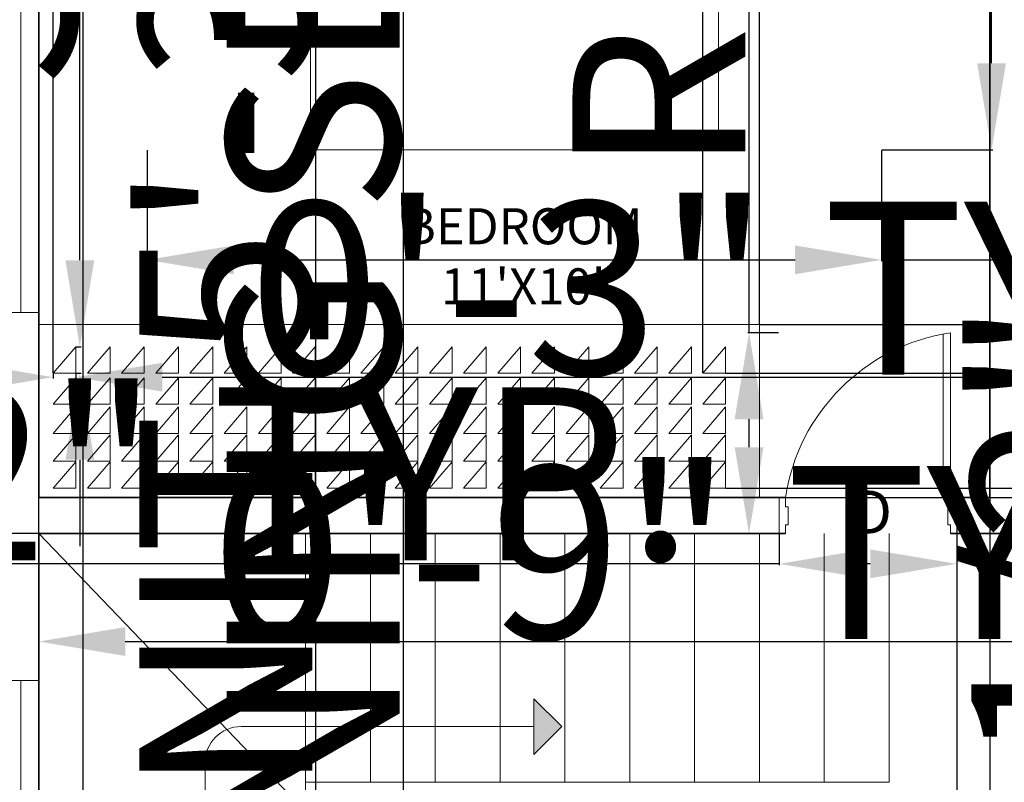
# Model space of a CAD drawing. Units: inches. Extents: x 2236 to 2927, y 1577 to 2452.
# Tile 5 of 9: x 2413 to 2550, y 1916 to 2021. Entities that reach past the tile are written whole.
import ezdxf

# ---------------------------------------------------------------- set-up
doc = ezdxf.new("R2010")
doc.units = ezdxf.units.IN
for name, color, linetype, lineweight in [('A-ANNO-DIMS', 2, 'Continuous', 18), ('A-ANNO-SYMB', 7, 'Continuous', 18), ('A-ANNO-TEXT', 7, 'Continuous', 18), ('A-AREA-IDEN', 7, 'Continuous', 18), ('A-FLOR-CASE', 40, 'Continuous', 18), ('A-FURN', 8, 'Continuous', 18), ('Doors', 150, 'Continuous', 18), ('Steps', 50, 'Continuous', 18), ('Wall', 7, 'Continuous', 35), ('Windows', 162, 'Continuous', 18)]:
    doc.layers.add(name, color=color, linetype=linetype, lineweight=lineweight)
doc.styles.get("Standard").update_dxf_attribs({"font": 'arial.ttf'})
doc.dimstyles.get("Standard").update_dxf_attribs({"dimtxt": 24, "dimasz": 12, "dimexe": 0.18, "dimexo": 0.0625, "dimgap": 0.09, "dimtad": 1, "dimdec": 1, "dimzin": 0, "dimdsep": 46, "dimlunit": 4, "dimtxsty": 'Standard', "dimcen": 0.09, "dimadec": 0, "dimazin": 0, "dimtfac": 1, "dimtdec": 1, "dimtofl": 0, "dimtmove": 0, "dimatfit": 3, "dimfxl": 1, "dimtolj": 1, "dimtzin": 0, "dimarcsym": 0})

# ---------------------------------------------------------------- blocks, each defined once
blk = doc.blocks.new('MAT-P13')
for p, q in [((-1.3496, 0), (-0.75, 0)), ((-1.3496, 0), (-1.3496, -0.2983)), ((-1.3496, -0.2983), (-0.75, 0)), ((-1.3496, 0), (-0.75, -0.2983)), ((-0.75, 0), (0.75, 0)), ((-0.75, 0), (-0.75, -1.9)), ((0.75, 0), (0.75, -1.9)), ((0.75, 0), (1.3496, 0)), ((1.3496, 0), (1.3496, -0.2983)), ((-0.7, -0.05), (-0.7, -0.35)), ((-0.7, -0.05), (-0.05, -0.05)), ((-0.05, -0.35), (-0.05, -0.05)), ((0.05, -0.05), (0.7, -0.05)), ((0.05, -0.35), (0.05, -0.05)), ((0.7, -0.05), (0.7, -0.35)), ((-0.75, -0.2983), (-1.3496, -0.2983)), ((1.3496, -0.2983), (0.75, -0.2983)), ((-0.7, -0.35), (-0.05, -0.35)), ((0.05, -0.35), (0.7, -0.35)), ((0, -0.4), (0.75, -0.398)), ((-0.75, -1.0034), (0, -0.4)), ((0, -0.4), (-0.75, -1.0034)), ((0, -0.4), (-0.2, -1.0034)), ((-0.75, -1.0034), (-0.2, -1.0034)), ((0.75, -1.9), (-0.75, -1.9))]:
    blk.add_line(p, q)
for radius in [0.1186, 0.0593]:
    blk.add_circle((1.0498, -0.1491), radius)
blk = doc.blocks.new('AP0B07')
for p, q in [((33.6, 96), (33.6, 978.8)), ((72, 96), (72, 972.3)), ((0, 96), (0, -96)), ((33.6, 96), (0, 96)), ((33.6, 48), (33.6, 96)), ((48, 48), (33.6, 48)), ((48, -48), (48, 48)), ((33.6, -96), (33.6, -48)), ((33.6, -48), (48, -48)), ((0, -96), (33.6, -96))]:
    blk.add_line(p, q)
blk.add_lwpolyline([(33.6, 96), (72, 96)])
blk.add_lwpolyline([(950, 96), (950, -96), (916.4, -96), (916.4, -48), (902, -48), (902, 48), (916.4, 48), (916.4, 96)], close=True)
blk.add_arc((-123.6, -61.2), 1051.8, 8.5964, 81.4036)
blk = doc.blocks.new('WIN-72IN')
for p, q in [((0, 6.5), (72, 6.5)), ((0, 4.5), (72, 4.5)), ((0, 2.5), (72, 2.5))]:
    blk.add_line(p, q)
blk.add_lwpolyline([(0, 9), (72, 9), (72, 0), (0, 0)], close=True)
blk = doc.blocks.new('WIN-36IN')
for p, q in [((2.5, 0), (2.5, 36)), ((4.5, 0), (4.5, 36)), ((6.5, 0), (6.5, 36))]:
    blk.add_line(p, q)
blk.add_lwpolyline([(0, 0), (0, 36), (9, 36), (9, 0)], close=True)
blk = doc.blocks.new('SHELF-TRIANGLE')
for p, q in [((3.15, 3.67), (0, 0)), ((3.15, 0), (3.15, 3.67)), ((0, 0), (3.15, 0))]:
    blk.add_line(p, q)
blk = doc.blocks.new('DIRECTION-ARROWHEAD')
h = blk.add_hatch(color=256)
h.dxf.hatch_style = 1
h.paths.add_polyline_path([(3.87, 3.87), (0, 7.74), (0, 0)])
for p, q in [((0, 7.74), (0, 0)), ((3.87, 3.87), (0, 7.74)), ((3.87, 3.87), (0, 0))]:
    blk.add_line(p, q)
blk = doc.blocks.new('*D16')
at = {"layer": 'A-ANNO-DIMS', "color": 0, "lineweight": -2, "transparency": 16777216}
for p, q in [((2421.54, 1988.01), (2421.54, 2451.93)), ((2421.05, 1976.01), (2421.72, 1976.01)), ((2421.05, 1972.34), (2421.72, 1972.34)), ((2421.54, 1960.34), (2421.54, 1948.34))]:
    blk.add_line(p, q, dxfattribs=at)
at = {"layer": 'A-ANNO-DIMS', "color": 0, "transparency": 16777216}
for points in [[(2419.54, 1988.01), (2423.54, 1988.01), (2421.54, 1976.01)], [(2419.54, 1960.34), (2423.54, 1960.34), (2421.54, 1972.34)]]:
    blk.add_solid(points, dxfattribs=at)
at = {"layer": 'Defpoints', "color": 0, "transparency": 16777216}
for p in [(2420.99, 1976.01), (2421.54, 1976.01), (2420.99, 1972.34)]:
    blk.add_point(p, dxfattribs=at)
at = {"layer": 'A-ANNO-DIMS', "color": 0, "transparency": 16777216, "insert": (2409.03, 2225.97), "char_height": 24, "attachment_point": 5, "rotation": 90}
blk.add_mtext('\\A1;SHELF INSERT 0\'-3 1/2" TYP.', dxfattribs=at)
blk = doc.blocks.new('*D17')
at = {"layer": 'A-ANNO-DIMS', "color": 0, "lineweight": -2, "transparency": 16777216}
for p, q in [((2417.85, 1972.28), (2417.85, 1971.61)), ((2420.99, 1972.28), (2420.99, 1971.61)), ((2405.85, 1971.79), (2393.85, 1971.79)), ((2432.99, 1971.79), (2591.46, 1971.79))]:
    blk.add_line(p, q, dxfattribs=at)
at = {"layer": 'A-ANNO-DIMS', "color": 0, "transparency": 16777216}
for points in [[(2405.85, 1973.79), (2405.85, 1969.79), (2417.85, 1971.79)], [(2432.99, 1973.79), (2432.99, 1969.79), (2420.99, 1971.79)]]:
    blk.add_solid(points, dxfattribs=at)
at = {"layer": 'Defpoints', "color": 0, "transparency": 16777216}
for p in [(2417.85, 1972.34), (2420.99, 1972.34), (2420.99, 1971.79)]:
    blk.add_point(p, dxfattribs=at)
at = {"layer": 'A-ANNO-DIMS', "color": 0, "transparency": 16777216, "insert": (2518.23, 1984.14), "char_height": 24, "attachment_point": 5}
blk.add_mtext('\\A1;0\'-3" TYP.', dxfattribs=at)
blk = doc.blocks.new('*D18')
at = {"layer": 'A-ANNO-DIMS', "color": 0, "lineweight": -2, "transparency": 16777216}
for p, q in [((2396.05, 1834.44), (2396.05, 2191.28)), ((2406.79, 1834.44), (2395.87, 1834.44)), ((2396.05, 1774.44), (2396.05, 1822.44)), ((2406.79, 1762.44), (2395.87, 1762.44))]:
    blk.add_line(p, q, dxfattribs=at)
at = {"layer": 'A-ANNO-DIMS', "color": 0, "transparency": 16777216}
for points in [[(2394.05, 1822.44), (2398.05, 1822.44), (2396.05, 1834.44)], [(2394.05, 1774.44), (2398.05, 1774.44), (2396.05, 1762.44)]]:
    blk.add_solid(points, dxfattribs=at)
at = {"layer": 'Defpoints', "color": 0, "transparency": 16777216}
for p in [(2396.05, 1834.44), (2406.85, 1834.44), (2406.85, 1762.44)]:
    blk.add_point(p, dxfattribs=at)
at = {"layer": 'A-ANNO-DIMS', "color": 0, "transparency": 16777216, "insert": (2383.54, 2018.86), "char_height": 24, "attachment_point": 5, "rotation": 90}
blk.add_mtext('\\A1;WINDOW W 6\'-0" TYP.', dxfattribs=at)
blk = doc.blocks.new('*D20')
at = {"layer": 'A-ANNO-DIMS', "color": 0, "lineweight": -2, "transparency": 16777216}
for p, q in [((2401.45, 1929.71), (2401.45, 2363.75)), ((2406.79, 1929.71), (2401.27, 1929.71)), ((2401.45, 1905.71), (2401.45, 1917.71)), ((2406.79, 1893.71), (2401.27, 1893.71))]:
    blk.add_line(p, q, dxfattribs=at)
at = {"layer": 'A-ANNO-DIMS', "color": 0, "transparency": 16777216}
for points in [[(2399.45, 1917.71), (2403.45, 1917.71), (2401.45, 1929.71)], [(2399.45, 1905.71), (2403.45, 1905.71), (2401.45, 1893.71)]]:
    blk.add_solid(points, dxfattribs=at)
at = {"layer": 'Defpoints', "color": 0, "transparency": 16777216}
for p in [(2401.45, 1929.71), (2406.85, 1929.71), (2406.85, 1893.71)]:
    blk.add_point(p, dxfattribs=at)
at = {"layer": 'A-ANNO-DIMS', "color": 0, "transparency": 16777216, "insert": (2388.93, 2152.73), "char_height": 24, "attachment_point": 5, "rotation": 90}
blk.add_mtext('\\A1;SMALL WINDOW 3\'-0" TYP.', dxfattribs=at)
blk = doc.blocks.new('*D21')
at = {"layer": 'A-ANNO-DIMS', "color": 0, "lineweight": -2, "transparency": 16777216}
for p, q in [((2394.85, 1935.11), (2382.85, 1935.11)), ((2406.85, 1929.77), (2406.85, 1935.29)), ((2415.85, 1929.77), (2415.85, 1935.29)), ((2427.85, 1935.11), (2586.32, 1935.11))]:
    blk.add_line(p, q, dxfattribs=at)
at = {"layer": 'A-ANNO-DIMS', "color": 0, "transparency": 16777216}
for points in [[(2394.85, 1937.11), (2394.85, 1933.11), (2406.85, 1935.11)], [(2427.85, 1937.11), (2427.85, 1933.11), (2415.85, 1935.11)]]:
    blk.add_solid(points, dxfattribs=at)
at = {"layer": 'Defpoints', "color": 0, "transparency": 16777216}
for p in [(2415.85, 1935.11), (2406.85, 1929.71), (2415.85, 1929.71)]:
    blk.add_point(p, dxfattribs=at)
at = {"layer": 'A-ANNO-DIMS', "color": 0, "transparency": 16777216, "insert": (2513.08, 1947.45), "char_height": 24, "attachment_point": 5}
blk.add_mtext('\\A1;0\'-9" TYP.', dxfattribs=at)
blk = doc.blocks.new('*D22')
at = {"layer": 'A-ANNO-DIMS', "color": 0, "lineweight": -2, "transparency": 16777216}
for p, q in [((2514.42, 1977.96), (2514.42, 2358.7)), ((2518.53, 1977.96), (2514.24, 1977.96)), ((2514.42, 1962.08), (2514.42, 1965.96)), ((2518.53, 1950.08), (2514.24, 1950.08))]:
    blk.add_line(p, q, dxfattribs=at)
at = {"layer": 'A-ANNO-DIMS', "color": 0, "transparency": 16777216}
for points in [[(2512.42, 1965.96), (2516.42, 1965.96), (2514.42, 1977.96)], [(2512.42, 1962.08), (2516.42, 1962.08), (2514.42, 1950.08)]]:
    blk.add_solid(points, dxfattribs=at)
at = {"layer": 'Defpoints', "color": 0, "transparency": 16777216}
for p in [(2514.42, 1977.96), (2518.6, 1977.96), (2518.6, 1950.08)]:
    blk.add_point(p, dxfattribs=at)
at = {"layer": 'A-ANNO-DIMS', "color": 0, "transparency": 16777216, "insert": (2501.91, 2174.33), "char_height": 24, "attachment_point": 5, "rotation": 90}
blk.add_mtext('\\A1;ROOM DOOR 2\'-4" TYP.', dxfattribs=at)
blk = doc.blocks.new('*D23')
at = {"layer": 'A-ANNO-DIMS', "color": 0, "lineweight": -2, "transparency": 16777216}
for p, q in [((2518.6, 1950.01), (2518.6, 1945.71)), ((2543.24, 1950.01), (2543.24, 1945.71)), ((2518.6, 1945.89), (2303.79, 1945.89)), ((2531.24, 1945.89), (2530.6, 1945.89))]:
    blk.add_line(p, q, dxfattribs=at)
at = {"layer": 'A-ANNO-DIMS', "color": 0, "transparency": 16777216}
for points in [[(2530.6, 1947.89), (2530.6, 1943.89), (2518.6, 1945.89)], [(2531.24, 1947.89), (2531.24, 1943.89), (2543.24, 1945.89)]]:
    blk.add_solid(points, dxfattribs=at)
at = {"layer": 'Defpoints', "color": 0, "transparency": 16777216}
for p in [(2518.6, 1950.08), (2543.24, 1950.08), (2518.6, 1945.89)]:
    blk.add_point(p, dxfattribs=at)
at = {"layer": 'A-ANNO-DIMS', "color": 0, "transparency": 16777216, "insert": (2405.19, 1958.39), "char_height": 24, "attachment_point": 5}
blk.add_mtext('\\A1;2\'-0 1/2" TYP.', dxfattribs=at)
blk = doc.blocks.new('*D28')
at = {"layer": 'A-ANNO-DIMS', "color": 0, "lineweight": -2, "transparency": 16777216}
for p, q in [((2430.9, 2003.29), (2430.9, 1987.89)), ((2532.8, 2003.29), (2532.8, 1987.89)), ((2442.9, 1988.07), (2520.8, 1988.07)), ((2532.8, 1988.07), (2818.23, 1988.07))]:
    blk.add_line(p, q, dxfattribs=at)
at = {"layer": 'A-ANNO-DIMS', "color": 0, "transparency": 16777216}
for points in [[(2442.9, 1990.07), (2442.9, 1986.07), (2430.9, 1988.07)], [(2520.8, 1990.07), (2520.8, 1986.07), (2532.8, 1988.07)]]:
    blk.add_solid(points, dxfattribs=at)
at = {"layer": 'Defpoints', "color": 0, "transparency": 16777216}
for p in [(2430.9, 2003.35), (2532.8, 2003.35), (2532.8, 1988.07)]:
    blk.add_point(p, dxfattribs=at)
at = {"layer": 'A-ANNO-DIMS', "color": 0, "transparency": 16777216, "insert": (2681.51, 2000.57), "char_height": 24, "attachment_point": 5}
blk.add_mtext('\\A1;BED GROUP 8\'-6"', dxfattribs=at)
blk = doc.blocks.new('*D29')
at = {"layer": 'A-ANNO-DIMS', "color": 0, "lineweight": -2, "transparency": 16777216}
for p, q in [((2548.08, 2075.08), (2548.08, 2225.62)), ((2532.86, 2075.08), (2548.26, 2075.08)), ((2548.08, 2015.35), (2548.08, 2063.08)), ((2532.86, 2003.35), (2548.26, 2003.35))]:
    blk.add_line(p, q, dxfattribs=at)
at = {"layer": 'A-ANNO-DIMS', "color": 0, "transparency": 16777216}
for points in [[(2546.08, 2063.08), (2550.08, 2063.08), (2548.08, 2075.08)], [(2546.08, 2015.35), (2550.08, 2015.35), (2548.08, 2003.35)]]:
    blk.add_solid(points, dxfattribs=at)
at = {"layer": 'Defpoints', "color": 0, "transparency": 16777216}
for p in [(2532.8, 2075.08), (2548.08, 2075.08), (2532.8, 2003.35)]:
    blk.add_point(p, dxfattribs=at)
at = {"layer": 'A-ANNO-DIMS', "color": 0, "transparency": 16777216, "insert": (2535.58, 2156.35), "char_height": 24, "attachment_point": 5, "rotation": 90}
blk.add_mtext('\\A1;5\'-11 1/2"', dxfattribs=at)
blk = doc.blocks.new('*D35')
at = {"layer": 'A-ANNO-DIMS', "color": 0, "lineweight": -2, "transparency": 16777216}
for p, q in [((2569.75, 1828.98), (2569.75, 1977.27)), ((2563.41, 1816.98), (2569.93, 1816.98)), ((2563.41, 1794.5), (2569.93, 1794.5)), ((2569.75, 1782.5), (2569.75, 1770.5))]:
    blk.add_line(p, q, dxfattribs=at)
at = {"layer": 'A-ANNO-DIMS', "color": 0, "transparency": 16777216}
for points in [[(2567.75, 1828.98), (2571.75, 1828.98), (2569.75, 1816.98)], [(2567.75, 1782.5), (2571.75, 1782.5), (2569.75, 1794.5)]]:
    blk.add_solid(points, dxfattribs=at)
at = {"layer": 'Defpoints', "color": 0, "transparency": 16777216}
for p in [(2563.35, 1816.98), (2569.75, 1816.98), (2563.35, 1794.5)]:
    blk.add_point(p, dxfattribs=at)
at = {"layer": 'A-ANNO-DIMS', "color": 0, "transparency": 16777216, "insert": (2557.25, 1909.13), "char_height": 24, "attachment_point": 5, "rotation": 90}
blk.add_mtext('\\A1;1\'-10 1/2"', dxfattribs=at)
blk = doc.blocks.new('*D36')
at = {"layer": 'A-ANNO-DIMS', "color": 0, "lineweight": -2, "transparency": 16777216}
for p, q in [((2454.3, 1796.23), (2454.3, 2047.2)), ((2444.91, 1796.23), (2454.48, 1796.23)), ((2454.3, 1745.23), (2454.3, 1784.23)), ((2444.91, 1733.23), (2454.48, 1733.23))]:
    blk.add_line(p, q, dxfattribs=at)
at = {"layer": 'A-ANNO-DIMS', "color": 0, "transparency": 16777216}
for points in [[(2452.3, 1784.23), (2456.3, 1784.23), (2454.3, 1796.23)], [(2452.3, 1745.23), (2456.3, 1745.23), (2454.3, 1733.23)]]:
    blk.add_solid(points, dxfattribs=at)
at = {"layer": 'Defpoints', "color": 0, "transparency": 16777216}
for p in [(2444.85, 1796.23), (2454.3, 1796.23), (2444.85, 1733.23)]:
    blk.add_point(p, dxfattribs=at)
at = {"layer": 'A-ANNO-DIMS', "color": 0, "transparency": 16777216, "insert": (2441.79, 1927.72), "char_height": 24, "attachment_point": 5, "rotation": 90}
blk.add_mtext('\\A1;SINK UNIT 5\'-3"', dxfattribs=at)
blk = doc.blocks.new('*D38')
at = {"layer": 'A-ANNO-DIMS', "color": 0, "lineweight": -2, "transparency": 16777216}
for p, q in [((2466.44, 1860.06), (2466.44, 2154.67)), ((2457.67, 1860.06), (2466.62, 1860.06)), ((2466.44, 1813.15), (2466.44, 1848.06)), ((2457.67, 1801.15), (2466.62, 1801.15))]:
    blk.add_line(p, q, dxfattribs=at)
at = {"layer": 'A-ANNO-DIMS', "color": 0, "transparency": 16777216}
for points in [[(2464.44, 1848.06), (2468.44, 1848.06), (2466.44, 1860.06)], [(2464.44, 1813.15), (2468.44, 1813.15), (2466.44, 1801.15)]]:
    blk.add_solid(points, dxfattribs=at)
at = {"layer": 'Defpoints', "color": 0, "transparency": 16777216}
for p in [(2457.61, 1860.06), (2466.44, 1860.06), (2457.61, 1801.15)]:
    blk.add_point(p, dxfattribs=at)
at = {"layer": 'A-ANNO-DIMS', "color": 0, "transparency": 16777216, "insert": (2453.94, 2013.36), "char_height": 24, "attachment_point": 5, "rotation": 90}
blk.add_mtext('\\A1;DINING SET 4\'-11"', dxfattribs=at)
blk = doc.blocks.new('*D39')
at = {"layer": 'A-ANNO-DIMS', "color": 0, "lineweight": -2, "transparency": 16777216}
for p, q in [((2422.01, 1868.89), (2271.05, 1868.89)), ((2422.01, 1860.12), (2422.01, 1869.07)), ((2445.61, 1868.89), (2434.01, 1868.89)), ((2457.61, 1860.12), (2457.61, 1869.07))]:
    blk.add_line(p, q, dxfattribs=at)
at = {"layer": 'A-ANNO-DIMS', "color": 0, "transparency": 16777216}
for points in [[(2434.01, 1870.89), (2434.01, 1866.89), (2422.01, 1868.89)], [(2445.61, 1870.89), (2445.61, 1866.89), (2457.61, 1868.89)]]:
    blk.add_solid(points, dxfattribs=at)
at = {"layer": 'Defpoints', "color": 0, "transparency": 16777216}
for p in [(2422.01, 1868.89), (2422.01, 1860.06), (2457.61, 1860.06)]:
    blk.add_point(p, dxfattribs=at)
at = {"layer": 'A-ANNO-DIMS', "color": 0, "transparency": 16777216, "insert": (2340.53, 1881.39), "char_height": 24, "attachment_point": 5}
blk.add_mtext('\\A1;2\'-11 1/2"', dxfattribs=at)
blk = doc.blocks.new('*D47')
at = {"layer": 'A-ANNO-DIMS', "color": 0, "lineweight": -2, "transparency": 16777216}
for p, q in [((2415.79, 1950.08), (2384.92, 1950.08)), ((2385.1, 1885.08), (2385.1, 1938.08)), ((2415.79, 1873.08), (2384.92, 1873.08))]:
    blk.add_line(p, q, dxfattribs=at)
at = {"layer": 'A-ANNO-DIMS', "color": 0, "transparency": 16777216}
for points in [[(2383.1, 1938.08), (2387.1, 1938.08), (2385.1, 1950.08)], [(2383.1, 1885.08), (2387.1, 1885.08), (2385.1, 1873.08)]]:
    blk.add_solid(points, dxfattribs=at)
at = {"layer": 'Defpoints', "color": 0, "transparency": 16777216}
for p in [(2385.1, 1950.08), (2415.85, 1950.08), (2415.85, 1873.08)]:
    blk.add_point(p, dxfattribs=at)
at = {"layer": 'A-ANNO-DIMS', "color": 0, "transparency": 16777216, "insert": (2372.75, 1911.58), "char_height": 24, "attachment_point": 5, "rotation": 90}
blk.add_mtext('\\A1;6\'-5"', dxfattribs=at)
blk = doc.blocks.new('*D51')
at = {"layer": 'A-ANNO-DIMS', "color": 0, "lineweight": -2, "transparency": 16777216}
for p, q in [((2644.6, 1862.15), (2644.6, 1994.46)), ((2512.91, 1862.15), (2644.78, 1862.15)), ((2644.6, 1847.53), (2644.6, 1850.15)), ((2512.91, 1835.53), (2644.78, 1835.53))]:
    blk.add_line(p, q, dxfattribs=at)
at = {"layer": 'A-ANNO-DIMS', "color": 0, "transparency": 16777216}
for points in [[(2642.6, 1850.15), (2646.6, 1850.15), (2644.6, 1862.15)], [(2642.6, 1847.53), (2646.6, 1847.53), (2644.6, 1835.53)]]:
    blk.add_solid(points, dxfattribs=at)
at = {"layer": 'Defpoints', "color": 0, "transparency": 16777216}
for p in [(2512.85, 1862.15), (2644.6, 1862.15), (2512.85, 1835.53)]:
    blk.add_point(p, dxfattribs=at)
at = {"layer": 'A-ANNO-DIMS', "color": 0, "transparency": 16777216, "insert": (2632.1, 1934.31), "char_height": 24, "attachment_point": 5, "rotation": 90}
blk.add_mtext('\\A1;2\'-2 1/2"', dxfattribs=at)
blk = doc.blocks.new('*D52')
at = {"layer": 'A-ANNO-DIMS', "color": 0, "lineweight": -2, "transparency": 16777216}
for p, q in [((2415.85, 1979.14), (2415.85, 2106.01)), ((2515.88, 1979.14), (2515.88, 2106.01)), ((2427.85, 2105.83), (2503.88, 2105.83))]:
    blk.add_line(p, q, dxfattribs=at)
at = {"layer": 'A-ANNO-DIMS', "color": 0, "transparency": 16777216}
for points in [[(2427.85, 2107.83), (2427.85, 2103.83), (2415.85, 2105.83)], [(2503.88, 2107.83), (2503.88, 2103.83), (2515.88, 2105.83)]]:
    blk.add_solid(points, dxfattribs=at)
at = {"layer": 'Defpoints', "color": 0, "transparency": 16777216}
for p in [(2515.88, 2105.83), (2415.85, 1979.08), (2515.88, 1979.08)]:
    blk.add_point(p, dxfattribs=at)
at = {"layer": 'A-ANNO-DIMS', "color": 0, "transparency": 16777216, "insert": (2465.87, 2118.17), "char_height": 24, "attachment_point": 5}
blk.add_mtext('\\A1;8\'-4"', dxfattribs=at)
blk = doc.blocks.new('*D53')
at = {"layer": 'A-ANNO-DIMS', "color": 0, "lineweight": -2, "transparency": 16777216}
for p, q in [((2644.6, 1991.08), (2644.6, 2067.46)), ((2515.94, 1979.08), (2644.78, 1979.08)), ((2515.94, 1955.08), (2644.78, 1955.08)), ((2644.6, 1943.08), (2644.6, 1931.08))]:
    blk.add_line(p, q, dxfattribs=at)
at = {"layer": 'A-ANNO-DIMS', "color": 0, "transparency": 16777216}
for points in [[(2642.6, 1991.08), (2646.6, 1991.08), (2644.6, 1979.08)], [(2642.6, 1943.08), (2646.6, 1943.08), (2644.6, 1955.08)]]:
    blk.add_solid(points, dxfattribs=at)
at = {"layer": 'Defpoints', "color": 0, "transparency": 16777216}
for p in [(2515.88, 1979.08), (2644.6, 1979.08), (2515.88, 1955.08)]:
    blk.add_point(p, dxfattribs=at)
at = {"layer": 'A-ANNO-DIMS', "color": 0, "transparency": 16777216, "insert": (2632.25, 2035.27), "char_height": 24, "attachment_point": 5, "rotation": 90}
blk.add_mtext('\\A1;2\'-0"', dxfattribs=at)
blk = doc.blocks.new('*D54')
at = {"layer": 'A-ANNO-DIMS', "color": 0, "lineweight": -2, "transparency": 16777216}
for p, q in [((2543.24, 1954.99), (2543.24, 1702.15)), ((2547.85, 1955.01), (2547.85, 1702.15)), ((2531.24, 1702.33), (2519.24, 1702.33)), ((2559.85, 1702.33), (2691.75, 1702.33))]:
    blk.add_line(p, q, dxfattribs=at)
at = {"layer": 'A-ANNO-DIMS', "color": 0, "transparency": 16777216}
for points in [[(2531.24, 1704.33), (2531.24, 1700.33), (2543.24, 1702.33)], [(2559.85, 1704.33), (2559.85, 1700.33), (2547.85, 1702.33)]]:
    blk.add_solid(points, dxfattribs=at)
at = {"layer": 'Defpoints', "color": 0, "transparency": 16777216}
for p in [(2543.24, 1955.06), (2547.85, 1955.08), (2547.85, 1702.33)]:
    blk.add_point(p, dxfattribs=at)
at = {"layer": 'A-ANNO-DIMS', "color": 0, "transparency": 16777216, "insert": (2631.8, 1714.83), "char_height": 24, "attachment_point": 5}
blk.add_mtext('\\A1;0\'-4 1/2"', dxfattribs=at)
blk = doc.blocks.new('*D60')
at = {"layer": 'A-ANNO-DIMS', "color": 0, "lineweight": -2, "transparency": 16777216}
for p, q in [((2385.1, 1881.08), (2385.1, 1957.05)), ((2415.79, 1869.08), (2384.92, 1869.08)), ((2434.57, 1860.06), (2384.92, 1860.06)), ((2385.1, 1848.06), (2385.1, 1836.06))]:
    blk.add_line(p, q, dxfattribs=at)
at = {"layer": 'A-ANNO-DIMS', "color": 0, "transparency": 16777216}
for points in [[(2383.1, 1881.08), (2387.1, 1881.08), (2385.1, 1869.08)], [(2383.1, 1848.06), (2387.1, 1848.06), (2385.1, 1860.06)]]:
    blk.add_solid(points, dxfattribs=at)
at = {"layer": 'Defpoints', "color": 0, "transparency": 16777216}
for p in [(2385.1, 1869.08), (2415.85, 1869.08), (2434.63, 1860.06)]:
    blk.add_point(p, dxfattribs=at)
at = {"layer": 'A-ANNO-DIMS', "color": 0, "transparency": 16777216, "insert": (2372.75, 1925.07), "char_height": 24, "attachment_point": 5, "rotation": 90}
blk.add_mtext('\\A1;0\'-9"', dxfattribs=at)
blk = doc.blocks.new('*D61')
at = {"layer": 'A-ANNO-DIMS', "color": 0, "lineweight": -2, "transparency": 16777216}
for p, q in [((2415.85, 1869.14), (2415.85, 2106.01)), ((2422.01, 1844.91), (2422.01, 2106.01)), ((2403.85, 2105.83), (2327.87, 2105.83)), ((2434.01, 2105.83), (2446.01, 2105.83))]:
    blk.add_line(p, q, dxfattribs=at)
at = {"layer": 'A-ANNO-DIMS', "color": 0, "transparency": 16777216}
for points in [[(2403.85, 2107.83), (2403.85, 2103.83), (2415.85, 2105.83)], [(2434.01, 2107.83), (2434.01, 2103.83), (2422.01, 2105.83)]]:
    blk.add_solid(points, dxfattribs=at)
at = {"layer": 'Defpoints', "color": 0, "transparency": 16777216}
for p in [(2415.85, 2105.83), (2415.85, 1869.08), (2422.01, 1844.84)]:
    blk.add_point(p, dxfattribs=at)
at = {"layer": 'A-ANNO-DIMS', "color": 0, "transparency": 16777216, "insert": (2359.86, 2118.17), "char_height": 24, "attachment_point": 5}
blk.add_mtext('\\A1;0\'-6"', dxfattribs=at)
blk = doc.blocks.new('*D62')
at = {"layer": 'A-ANNO-DIMS', "color": 0, "lineweight": -2, "transparency": 16777216}
for p, q in [((2417.85, 1972.4), (2417.85, 2106.01)), ((2508.01, 1972.4), (2508.01, 2106.01)), ((2429.85, 2105.83), (2496.01, 2105.83))]:
    blk.add_line(p, q, dxfattribs=at)
at = {"layer": 'A-ANNO-DIMS', "color": 0, "transparency": 16777216}
for points in [[(2429.85, 2107.83), (2429.85, 2103.83), (2417.85, 2105.83)], [(2496.01, 2107.83), (2496.01, 2103.83), (2508.01, 2105.83)]]:
    blk.add_solid(points, dxfattribs=at)
at = {"layer": 'Defpoints', "color": 0, "transparency": 16777216}
for p in [(2508.01, 2105.83), (2417.85, 1972.34), (2508.01, 1972.34)]:
    blk.add_point(p, dxfattribs=at)
at = {"layer": 'A-ANNO-DIMS', "color": 0, "transparency": 16777216, "insert": (2462.93, 2118.17), "char_height": 24, "attachment_point": 5}
blk.add_mtext('\\A1;7\'-6"', dxfattribs=at)
blk = doc.blocks.new('*D63')
at = {"layer": 'A-ANNO-DIMS', "color": 0, "lineweight": -2, "transparency": 16777216}
for p, q in [((2644.6, 1984.34), (2644.6, 2058.06)), ((2511.22, 1972.34), (2644.78, 1972.34)), ((2511.22, 1956.39), (2644.78, 1956.39)), ((2644.6, 1944.39), (2644.6, 1932.39))]:
    blk.add_line(p, q, dxfattribs=at)
at = {"layer": 'A-ANNO-DIMS', "color": 0, "transparency": 16777216}
for points in [[(2642.6, 1984.34), (2646.6, 1984.34), (2644.6, 1972.34)], [(2642.6, 1944.39), (2646.6, 1944.39), (2644.6, 1956.39)]]:
    blk.add_solid(points, dxfattribs=at)
at = {"layer": 'Defpoints', "color": 0, "transparency": 16777216}
for p in [(2511.16, 1972.34), (2644.6, 1972.34), (2511.16, 1956.39)]:
    blk.add_point(p, dxfattribs=at)
at = {"layer": 'A-ANNO-DIMS', "color": 0, "transparency": 16777216, "insert": (2632.46, 2027.2), "char_height": 24, "attachment_point": 5, "rotation": 90}
blk.add_mtext('\\A1;1\'-4"', dxfattribs=at)

msp = doc.modelspace()

# ---------------------------------------------------------------- linework, layer by layer
at = {"layer": 'A-ANNO-SYMB'}
for p, q in [((2443.92, 1923.31), (2484.55, 1923.31)), ((2438.92, 1901.13), (2438.92, 1918.31))]:
    msp.add_line(p, q, dxfattribs=at)
msp.add_arc((2443.92, 1918.31), 5, 90, 180, dxfattribs=at)
at = {"layer": 'A-FLOR-CASE'}
for p in [(2415.85, 1979.08), (2515.88, 1955.08)]:
    msp.add_line(p, (2515.88, 1979.08), dxfattribs=at)
at = {"layer": 'Steps'}
for p, q in [((2452.86, 1911.58), (2415.85, 1950.08)), ((2452.86, 1873.08), (2452.86, 1950.08)), ((2461.86, 1915.58), (2461.86, 1950.08)), ((2470.86, 1915.58), (2470.86, 1950.08)), ((2479.86, 1915.58), (2479.86, 1950.08)), ((2488.86, 1915.58), (2488.86, 1950.08)), ((2497.86, 1915.58), (2497.86, 1950.08)), ((2506.86, 1915.58), (2506.86, 1950.08)), ((2515.86, 1915.58), (2515.86, 1950.08)), ((2524.86, 1915.58), (2524.86, 1950.08)), ((2533.86, 1915.58), (2533.86, 1950.08)), ((2533.86, 1915.58), (2452.86, 1915.58))]:
    msp.add_line(p, q, dxfattribs=at)
at = {"layer": 'Wall'}
for p, q in [((2415.85, 2075.08), (2415.85, 1955.08)), ((2547.85, 2075.08), (2547.85, 1955.08)), ((2415.85, 1955.08), (2519.47, 1955.08)), ((2541.37, 1955.08), (2547.85, 1955.08)), ((2415.85, 1950.08), (2519.47, 1950.08)), ((2415.85, 1950.08), (2415.85, 1873.08)), ((2542.37, 1950.08), (2551.85, 1950.08))]:
    msp.add_line(p, q, dxfattribs=at)

# ---------------------------------------------------------------- block references
at = {"layer": 'A-ANNO-SYMB'}
msp.add_blockref('DIRECTION-ARROWHEAD', (2484.55, 1919.44), dxfattribs=at)
at = {"layer": 'A-FLOR-CASE'}
for p in [(2417.85, 1972.34), (2422.59, 1972.34), (2427.34, 1972.34), (2432.08, 1972.34), (2436.83, 1972.34), (2441.57, 1972.34), (2446.32, 1972.34), (2451.07, 1972.34), (2455.81, 1972.34), (2460.56, 1972.34), (2465.3, 1972.34), (2470.05, 1972.34), (2474.79, 1972.34), (2479.54, 1972.34), (2484.28, 1972.34), (2489.03, 1972.34), (2493.78, 1972.34), (2498.52, 1972.34), (2503.27, 1972.34), (2508.01, 1972.34), (2417.85, 1968.05), (2422.59, 1968.05), (2427.34, 1968.05), (2432.08, 1968.05), (2436.83, 1968.05), (2441.57, 1968.05), (2446.32, 1968.05), (2451.07, 1968.05), (2455.81, 1968.05), (2460.56, 1968.05), (2465.3, 1968.05), (2470.05, 1968.05), (2474.79, 1968.05), (2479.54, 1968.05), (2484.28, 1968.05), (2489.03, 1968.05), (2493.78, 1968.05), (2498.52, 1968.05), (2503.27, 1968.05), (2508.01, 1968.05), (2417.85, 1963.99), (2422.59, 1963.99), (2427.34, 1963.99), (2432.08, 1963.99), (2436.83, 1963.99), (2441.57, 1963.99), (2446.32, 1963.99), (2451.07, 1963.99), (2455.81, 1963.99), (2460.56, 1963.99), (2465.3, 1963.99), (2470.05, 1963.99), (2474.79, 1963.99), (2479.54, 1963.99), (2484.28, 1963.99), (2489.03, 1963.99), (2493.78, 1963.99), (2498.52, 1963.99), (2503.27, 1963.99), (2508.01, 1963.99), (2417.85, 1960.13), (2422.59, 1960.13), (2427.34, 1960.13), (2432.08, 1960.13), (2436.83, 1960.13), (2441.57, 1960.13), (2446.32, 1960.13), (2451.07, 1960.13), (2455.81, 1960.13), (2460.56, 1960.13), (2465.3, 1960.13), (2470.05, 1960.13), (2474.79, 1960.13), (2479.54, 1960.13), (2484.28, 1960.13), (2489.03, 1960.13), (2493.78, 1960.13), (2498.52, 1960.13), (2503.27, 1960.13), (2508.01, 1960.13), (2417.85, 1956.39), (2422.59, 1956.39), (2427.34, 1956.39), (2432.08, 1956.39), (2436.83, 1956.39), (2441.57, 1956.39), (2446.32, 1956.39), (2451.07, 1956.39), (2455.81, 1956.39), (2460.56, 1956.39), (2465.3, 1956.39), (2470.05, 1956.39), (2474.79, 1956.39), (2479.54, 1956.39), (2484.28, 1956.39), (2489.03, 1956.39), (2493.78, 1956.39), (2498.52, 1956.39), (2503.27, 1956.39), (2508.01, 1956.39)]:
    msp.add_blockref('SHELF-TRIANGLE', p, dxfattribs=at)
at = {"layer": 'A-FURN', "xscale": 37.75073971806934, "yscale": 37.75073971806934, "zscale": 37.75073971806934}
msp.add_blockref('MAT-P13', (2481.85, 2075.08), dxfattribs=at)
at = {"layer": 'Doors', "xscale": -0.0259404460783577, "yscale": 0.0259404460783577, "zscale": 0.0259404460783577}
msp.add_blockref('AP0B07', (2543.24, 1952.57), dxfattribs=at)
at = {"layer": 'Windows', "rotation": 90.00000000000261}
msp.add_blockref('WIN-72IN', (2415.85, 1980.78), dxfattribs=at)
at = {"layer": 'Windows'}
msp.add_blockref('WIN-36IN', (2406.85, 1893.71), dxfattribs=at)

# ---------------------------------------------------------------- texts
at = {"layer": 'A-ANNO-TEXT'}
msp.add_text('D', height=6, dxfattribs=at).set_placement((2528.64, 1950.08))
at = {"layer": 'A-AREA-IDEN', "insert": (2464.35, 1995.23), "char_height": 5, "attachment_point": 1}
msp.add_mtext_dynamic_manual_height_columns("\\pxqc;BEDROOM\\P11'X10'", width=37.4353, gutter_width=12.5, heights=[0], dxfattribs=at)

# ---------------------------------------------------------------- dimensions: what is measured, and where the dimension line sits
at = {"layer": 'A-ANNO-DIMS'}
for base, p1, p2, angle, text, picture, middle in [((2421.54, 1976.01), (2420.99, 1972.34), (2420.99, 1976.01), 90, 'SHELF INSERT <> TYP.', '*D16', (2409.03, 2225.97)), ((2401.45, 1929.71), (2406.85, 1893.71), (2406.85, 1929.71), 90, 'SMALL WINDOW <> TYP.', '*D20', (2388.93, 2152.73)), ((2514.42, 1977.96), (2518.6, 1950.08), (2518.6, 1977.96), 90, 'ROOM DOOR <> TYP.', '*D22', (2501.91, 2174.33)), ((2396.05, 1834.44), (2406.85, 1762.44), (2406.85, 1834.44), 90, 'WINDOW W <> TYP.', '*D18', (2383.54, 2018.86)), ((2466.44, 1860.06), (2457.61, 1801.15), (2457.61, 1860.06), 90, 'DINING SET <>', '*D38', (2453.94, 2013.36)), ((2454.3, 1796.23), (2444.85, 1733.23), (2444.85, 1796.23), 90, 'SINK UNIT <>', '*D36', (2441.79, 1927.72)), ((2518.6, 1945.89), (2543.24, 1950.08), (2518.6, 1950.08), 180, '<> TYP.', '*D23', (2405.19, 1958.39))]:
    dim = msp.add_linear_dim(base=base, p1=p1, p2=p2, angle=angle, text=text, dimstyle='Standard', override={"dimdec": 1, "dimlfac": 1, "dimrnd": 0, "dimzin": 1, "dimdsep": 46, "dimlunit": 4, "dimfrac": 2}, dxfattribs=at)
    dim.commit()
    dim.dimension.update_dxf_attribs({"geometry": picture, "text_midpoint": middle})
for base, p1, p2, angle, picture, middle in [((2548.08, 2075.08), (2532.8, 2003.35), (2532.8, 2075.08), 90, '*D29', (2535.58, 2156.35)), ((2644.6, 1979.08), (2515.88, 1955.08), (2515.88, 1979.08), 90, '*D53', (2632.25, 2035.27)), ((2644.598, 1972.3393), (2511.1585, 1956.3877), (2511.1585, 1972.3393), 90, '*D63', (2632.4589, 2027.1987)), ((2644.6, 1862.15), (2512.85, 1835.53), (2512.85, 1862.15), 90, '*D51', (2632.1, 1934.31)), ((2569.75, 1816.98), (2563.35, 1794.5), (2563.35, 1816.98), 90, '*D35', (2557.25, 1909.13)), ((2385.1, 1869.08), (2434.63, 1860.06), (2415.85, 1869.08), 90, '*D60', (2372.75, 1925.07)), ((2385.1, 1950.08), (2415.85, 1873.08), (2415.85, 1950.08), 90, '*D47', (2372.75, 1911.58)), ((2422.01, 1868.89), (2457.61, 1860.06), (2422.01, 1860.06), 180, '*D39', (2340.53, 1881.39))]:
    dim = msp.add_linear_dim(base=base, p1=p1, p2=p2, angle=angle, dimstyle='Standard', override={"dimdec": 1, "dimlfac": 1, "dimrnd": 0, "dimzin": 1, "dimdsep": 46, "dimlunit": 4, "dimfrac": 2}, dxfattribs=at)
    dim.commit()
    dim.dimension.update_dxf_attribs({"geometry": picture, "text_midpoint": middle})
for base, p1, p2, picture, middle in [((2415.85, 2105.83), (2422.01, 1844.84), (2415.85, 1869.08), '*D61', (2359.86, 2118.17)), ((2515.88, 2105.83), (2415.85, 1979.08), (2515.88, 1979.08), '*D52', (2465.87, 2118.17)), ((2508.01, 2105.83), (2417.85, 1972.34), (2508.01, 1972.34), '*D62', (2462.93, 2118.17)), ((2547.85, 1702.33), (2543.24, 1955.06), (2547.85, 1955.08), '*D54', (2631.8, 1714.83))]:
    dim = msp.add_linear_dim(base=base, p1=p1, p2=p2, dimstyle='Standard', override={"dimdec": 1, "dimlfac": 1, "dimrnd": 0, "dimzin": 1, "dimdsep": 46, "dimlunit": 4, "dimfrac": 2}, dxfattribs=at)
    dim.commit()
    dim.dimension.update_dxf_attribs({"geometry": picture, "text_midpoint": middle})
for base, p1, p2, text, picture, middle in [((2532.8, 1988.07), (2430.9, 2003.35), (2532.8, 2003.35), 'BED GROUP <>', '*D28', (2681.51, 2000.57)), ((2420.99, 1971.79), (2417.85, 1972.34), (2420.99, 1972.34), '<> TYP.', '*D17', (2518.23, 1984.14)), ((2415.85, 1935.11), (2406.85, 1929.71), (2415.85, 1929.71), '<> TYP.', '*D21', (2513.08, 1947.45))]:
    dim = msp.add_linear_dim(base=base, p1=p1, p2=p2, text=text, dimstyle='Standard', override={"dimdec": 1, "dimlfac": 1, "dimrnd": 0, "dimzin": 1, "dimdsep": 46, "dimlunit": 4, "dimfrac": 2}, dxfattribs=at)
    dim.commit()
    dim.dimension.update_dxf_attribs({"geometry": picture, "text_midpoint": middle})

doc.saveas('drawing.dxf')
